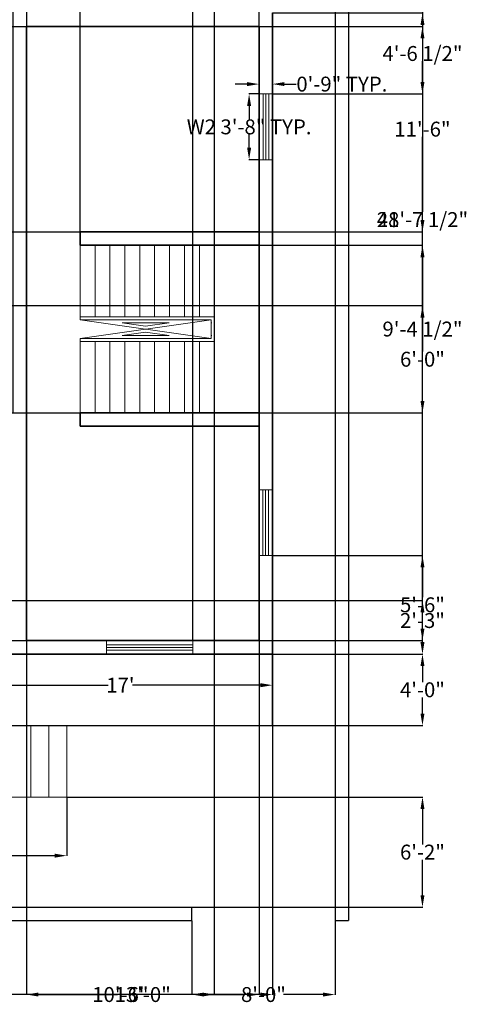
# Model space of a CAD drawing. Units: inches. Extents: x -63 to 800, y 3068 to 4133.
# Tile 3 of 5: x 501 to 800, y 3076 to 3737. Entities that reach past the tile are written whole.
import ezdxf

# ---------------------------------------------------------------- set-up
doc = ezdxf.new("R2010")
doc.units = ezdxf.units.IN
doc.header["$MEASUREMENT"] = 0
for name, color, linetype, lineweight in [('A-ANNO-DIMS', 2, 'Continuous', 13), ('A-FLOR', 7, 'Continuous', 25), ('A-FLOR-STRS', 3, 'Continuous', 18), ('A-GLAZ', 4, 'Continuous', 18), ('A-WALL', 7, 'Continuous', 35), ('A-WALL-SITE', 8, 'Continuous', 30)]:
    doc.layers.add(name, color=color, linetype=linetype, lineweight=lineweight)
doc.styles.get("Standard").update_dxf_attribs({"font": 'arial.ttf'})
doc.dimstyles.get("Standard").update_dxf_attribs({"dimtxt": 10, "dimasz": 8, "dimexe": 0.18, "dimexo": 0.0625, "dimgap": 0.09, "dimtad": 0, "dimtih": 1, "dimtoh": 1, "dimdec": 0, "dimzin": 0, "dimdsep": 46, "dimlunit": 3, "dimtxsty": 'Standard', "dimcen": 0.09, "dimadec": 0, "dimazin": 0, "dimtfac": 1, "dimtdec": 0, "dimtofl": 0, "dimtmove": 0, "dimatfit": 3, "dimfxl": 1, "dimtolj": 1, "dimtzin": 0, "dimarcsym": 0})

# ---------------------------------------------------------------- blocks, each defined once
blk = doc.blocks.new('*D7')
at = {"layer": 'A-ANNO-DIMS', "color": 0, "lineweight": -2, "transparency": 16777216}
for p, q in [((331.31, 3215.25), (331.31, 3175.73)), ((532.31, 3215.25), (532.31, 3175.73)), ((339.31, 3175.91), (415.01, 3175.91)), ((524.31, 3175.91), (448.6, 3175.91))]:
    blk.add_line(p, q, dxfattribs=at)
at = {"layer": 'A-ANNO-DIMS', "color": 0, "transparency": 16777216}
for points in [[(339.31, 3177.24), (339.31, 3174.58), (331.31, 3175.91)], [(524.31, 3177.24), (524.31, 3174.58), (532.31, 3175.91)]]:
    blk.add_solid(points, dxfattribs=at)
at = {"layer": 'Defpoints', "color": 0, "transparency": 16777216}
for p in [(331.31, 3215.31), (532.31, 3215.31), (532.31, 3175.91)]:
    blk.add_point(p, dxfattribs=at)
at = {"layer": 'A-ANNO-DIMS', "color": 0, "transparency": 16777216, "insert": (431.81, 3175.91), "char_height": 10, "attachment_point": 5}
blk.add_mtext('\\A1;16\'-9"', dxfattribs=at)
blk = doc.blocks.new('*D9')
at = {"layer": 'A-ANNO-DIMS', "color": 0, "lineweight": -2, "transparency": 16777216}
for p, q in [((466.31, 3287.37), (466.31, 3290.58)), ((474.31, 3290.4), (560.2, 3290.4)), ((662.31, 3290.4), (576.41, 3290.4)), ((670.31, 3287.37), (670.31, 3290.58))]:
    blk.add_line(p, q, dxfattribs=at)
at = {"layer": 'A-ANNO-DIMS', "color": 0, "transparency": 16777216}
for points in [[(474.31, 3291.73), (474.31, 3289.06), (466.31, 3290.4)], [(662.31, 3291.73), (662.31, 3289.06), (670.31, 3290.4)]]:
    blk.add_solid(points, dxfattribs=at)
at = {"layer": 'Defpoints', "color": 0, "transparency": 16777216}
for p in [(466.31, 3287.31), (670.31, 3290.4), (670.31, 3287.31)]:
    blk.add_point(p, dxfattribs=at)
at = {"layer": 'A-ANNO-DIMS', "color": 0, "transparency": 16777216, "insert": (568.31, 3290.4), "char_height": 10, "attachment_point": 5}
blk.add_mtext("\\A1;17'", dxfattribs=at)
blk = doc.blocks.new('WIN-44')
blk.add_lwpolyline([(0, 0), (0, 44.17), (9, 44.17), (9, 0)], close=True)
for points in [[(2.71, 44.17), (2.71, 0), (6.5, 0), (6.5, 44.17)], [(4.5, 0), (4.5, 44.17)]]:
    blk.add_lwpolyline(points)
blk = doc.blocks.new('WIN-58')
blk.add_lwpolyline([(0, 9), (57.99, 9), (57.99, 0), (0, 0)], close=True)
for points in [[(0, 4.5), (57.99, 4.5), (57.99, 6.29), (0, 6.29)], [(0, 2.51), (57.99, 2.51)]]:
    blk.add_lwpolyline(points)
blk = doc.blocks.new('*D15')
at = {"layer": 'A-ANNO-DIMS', "color": 0, "lineweight": -2, "transparency": 16777216}
for p, q in [((661.25, 3687.44), (654.5, 3687.44)), ((654.68, 3679.44), (654.68, 3670.55)), ((654.68, 3651.26), (654.68, 3660.15)), ((661.25, 3643.26), (654.5, 3643.26))]:
    blk.add_line(p, q, dxfattribs=at)
at = {"layer": 'A-ANNO-DIMS', "color": 0, "transparency": 16777216}
for points in [[(653.35, 3679.44), (656.02, 3679.44), (654.68, 3687.44)], [(653.35, 3651.26), (656.02, 3651.26), (654.68, 3643.26)]]:
    blk.add_solid(points, dxfattribs=at)
at = {"layer": 'Defpoints', "color": 0, "transparency": 16777216}
for p in [(654.68, 3687.44), (661.31, 3687.44), (661.31, 3643.26)]:
    blk.add_point(p, dxfattribs=at)
at = {"layer": 'A-ANNO-DIMS', "color": 0, "transparency": 16777216, "insert": (654.68, 3665.35), "char_height": 10, "attachment_point": 5}
blk.add_mtext('\\A1;W2 3\'-8" TYP.', dxfattribs=at)
blk = doc.blocks.new('*D16')
at = {"layer": 'A-ANNO-DIMS', "color": 0, "lineweight": -2, "transparency": 16777216}
for p, q in [((653.31, 3694.06), (645.31, 3694.06)), ((661.31, 3687.5), (661.31, 3694.24)), ((670.31, 3687.5), (670.31, 3694.24)), ((678.31, 3694.06), (686.31, 3694.06))]:
    blk.add_line(p, q, dxfattribs=at)
at = {"layer": 'A-ANNO-DIMS', "color": 0, "transparency": 16777216}
for points in [[(653.31, 3695.39), (653.31, 3692.73), (661.31, 3694.06)], [(678.31, 3695.39), (678.31, 3692.73), (670.31, 3694.06)]]:
    blk.add_solid(points, dxfattribs=at)
at = {"layer": 'Defpoints', "color": 0, "transparency": 16777216}
for p in [(670.31, 3694.06), (661.31, 3687.44), (670.31, 3687.44)]:
    blk.add_point(p, dxfattribs=at)
at = {"layer": 'A-ANNO-DIMS', "color": 0, "transparency": 16777216, "insert": (716.88, 3694.06), "char_height": 10, "attachment_point": 5}
blk.add_mtext('\\A1;0\'-9" TYP.', dxfattribs=at)
blk = doc.blocks.new('*D22')
at = {"layer": 'A-ANNO-DIMS', "color": 0, "lineweight": -2, "transparency": 16777216}
for p, q in [((616.31, 3132.25), (616.31, 3082.48)), ((712.31, 3132.25), (712.31, 3082.48)), ((624.31, 3082.66), (650.92, 3082.66)), ((704.31, 3082.66), (677.7, 3082.66))]:
    blk.add_line(p, q, dxfattribs=at)
at = {"layer": 'A-ANNO-DIMS', "color": 0, "transparency": 16777216}
for points in [[(624.31, 3083.99), (624.31, 3081.33), (616.31, 3082.66)], [(704.31, 3083.99), (704.31, 3081.33), (712.31, 3082.66)]]:
    blk.add_solid(points, dxfattribs=at)
at = {"layer": 'Defpoints', "color": 0, "transparency": 16777216}
for p in [(616.31, 3132.31), (712.31, 3132.31), (712.31, 3082.66)]:
    blk.add_point(p, dxfattribs=at)
at = {"layer": 'A-ANNO-DIMS', "color": 0, "transparency": 16777216, "insert": (664.31, 3082.66), "char_height": 10, "attachment_point": 5}
blk.add_mtext('\\A1;8\'-0"', dxfattribs=at)
blk = doc.blocks.new('*D33')
at = {"layer": 'A-ANNO-DIMS', "color": 0, "lineweight": -2, "transparency": 16777216}
for p, q in [((532.37, 3215.31), (771.14, 3215.31)), ((770.96, 3207.31), (770.96, 3183.51)), ((770.96, 3149.31), (770.96, 3173.11)), ((616.37, 3141.31), (771.14, 3141.31))]:
    blk.add_line(p, q, dxfattribs=at)
at = {"layer": 'A-ANNO-DIMS', "color": 0, "transparency": 16777216}
for points in [[(769.63, 3207.31), (772.29, 3207.31), (770.96, 3215.31)], [(769.63, 3149.31), (772.29, 3149.31), (770.96, 3141.31)]]:
    blk.add_solid(points, dxfattribs=at)
at = {"layer": 'Defpoints', "color": 0, "transparency": 16777216}
for p in [(532.31, 3215.31), (770.96, 3215.31), (616.31, 3141.31)]:
    blk.add_point(p, dxfattribs=at)
at = {"layer": 'A-ANNO-DIMS', "color": 0, "transparency": 16777216, "insert": (770.96, 3178.31), "char_height": 10, "attachment_point": 5}
blk.add_mtext('\\A1;6\'-2"', dxfattribs=at)
blk = doc.blocks.new('*D34')
at = {"layer": 'A-ANNO-DIMS', "color": 0, "lineweight": -2, "transparency": 16777216}
for p, q in [((142.31, 3522.75), (142.31, 3082.48)), ((670.31, 3263.25), (670.31, 3082.48)), ((150.31, 3082.66), (388.84, 3082.66)), ((662.31, 3082.66), (423.78, 3082.66))]:
    blk.add_line(p, q, dxfattribs=at)
at = {"layer": 'A-ANNO-DIMS', "color": 0, "transparency": 16777216}
for points in [[(150.31, 3083.99), (150.31, 3081.33), (142.31, 3082.66)], [(662.31, 3083.99), (662.31, 3081.33), (670.31, 3082.66)]]:
    blk.add_solid(points, dxfattribs=at)
at = {"layer": 'Defpoints', "color": 0, "transparency": 16777216}
for p in [(142.31, 3522.81), (670.31, 3263.31), (670.31, 3082.66)]:
    blk.add_point(p, dxfattribs=at)
at = {"layer": 'A-ANNO-DIMS', "color": 0, "transparency": 16777216, "insert": (406.31, 3082.66), "char_height": 10, "attachment_point": 5}
blk.add_mtext('\\A1;44\'-0"', dxfattribs=at)
blk = doc.blocks.new('*D35')
at = {"layer": 'A-ANNO-DIMS', "color": 0, "lineweight": -2, "transparency": 16777216}
for p, q in [((640.37, 3894.81), (771.14, 3894.81)), ((770.96, 3886.81), (770.96, 3608.32)), ((770.96, 3319.31), (770.96, 3597.8)), ((670.37, 3311.31), (771.14, 3311.31))]:
    blk.add_line(p, q, dxfattribs=at)
at = {"layer": 'A-ANNO-DIMS', "color": 0, "transparency": 16777216}
for points in [[(769.63, 3886.81), (772.29, 3886.81), (770.96, 3894.81)], [(769.63, 3319.31), (772.29, 3319.31), (770.96, 3311.31)]]:
    blk.add_solid(points, dxfattribs=at)
at = {"layer": 'Defpoints', "color": 0, "transparency": 16777216}
for p in [(640.31, 3894.81), (770.96, 3894.81), (670.31, 3311.31)]:
    blk.add_point(p, dxfattribs=at)
at = {"layer": 'A-ANNO-DIMS', "color": 0, "transparency": 16777216, "insert": (770.96, 3603.06), "char_height": 10, "attachment_point": 5}
blk.add_mtext('\\A1;48\'-7 1/2"', dxfattribs=at)
blk = doc.blocks.new('*D39')
at = {"layer": 'A-ANNO-DIMS', "color": 0, "lineweight": -2, "transparency": 16777216}
for p, q in [((505.31, 3885.75), (505.31, 3082.48)), ((631.31, 3885.75), (631.31, 3082.48)), ((513.31, 3082.66), (551.51, 3082.66)), ((623.31, 3082.66), (585.1, 3082.66))]:
    blk.add_line(p, q, dxfattribs=at)
at = {"layer": 'A-ANNO-DIMS', "color": 0, "transparency": 16777216}
for points in [[(513.31, 3083.99), (513.31, 3081.33), (505.31, 3082.66)], [(623.31, 3083.99), (623.31, 3081.33), (631.31, 3082.66)]]:
    blk.add_solid(points, dxfattribs=at)
at = {"layer": 'Defpoints', "color": 0, "transparency": 16777216}
for p in [(505.31, 3885.81), (631.31, 3885.81), (631.31, 3082.66)]:
    blk.add_point(p, dxfattribs=at)
at = {"layer": 'A-ANNO-DIMS', "color": 0, "transparency": 16777216, "insert": (568.31, 3082.66), "char_height": 10, "attachment_point": 5}
blk.add_mtext('\\A1;10\'-6"', dxfattribs=at)
blk = doc.blocks.new('*D46')
at = {"layer": 'A-ANNO-DIMS', "color": 0, "lineweight": -2, "transparency": 16777216}
for p, q in [((505.31, 3732.75), (505.31, 3082.48)), ((661.31, 3732.75), (661.31, 3082.48)), ((513.31, 3082.66), (566.51, 3082.66)), ((653.31, 3082.66), (600.1, 3082.66))]:
    blk.add_line(p, q, dxfattribs=at)
at = {"layer": 'A-ANNO-DIMS', "color": 0, "transparency": 16777216}
for points in [[(513.31, 3083.99), (513.31, 3081.33), (505.31, 3082.66)], [(653.31, 3083.99), (653.31, 3081.33), (661.31, 3082.66)]]:
    blk.add_solid(points, dxfattribs=at)
at = {"layer": 'Defpoints', "color": 0, "transparency": 16777216}
for p in [(505.31, 3732.81), (661.31, 3732.81), (661.31, 3082.66)]:
    blk.add_point(p, dxfattribs=at)
at = {"layer": 'A-ANNO-DIMS', "color": 0, "transparency": 16777216, "insert": (583.31, 3082.66), "char_height": 10, "attachment_point": 5}
blk.add_mtext('\\A1;13\'-0"', dxfattribs=at)
blk = doc.blocks.new('*D47')
at = {"layer": 'A-ANNO-DIMS', "color": 0, "lineweight": -2, "transparency": 16777216}
for p, q in [((151.37, 3732.81), (771.14, 3732.81)), ((770.96, 3724.81), (770.96, 3669.01)), ((770.96, 3602.81), (770.96, 3658.61)), ((151.37, 3594.81), (771.14, 3594.81))]:
    blk.add_line(p, q, dxfattribs=at)
at = {"layer": 'A-ANNO-DIMS', "color": 0, "transparency": 16777216}
for points in [[(769.63, 3724.81), (772.29, 3724.81), (770.96, 3732.81)], [(769.63, 3602.81), (772.29, 3602.81), (770.96, 3594.81)]]:
    blk.add_solid(points, dxfattribs=at)
at = {"layer": 'Defpoints', "color": 0, "transparency": 16777216}
for p in [(151.31, 3732.81), (770.96, 3732.81), (151.31, 3594.81)]:
    blk.add_point(p, dxfattribs=at)
at = {"layer": 'A-ANNO-DIMS', "color": 0, "transparency": 16777216, "insert": (770.96, 3663.81), "char_height": 10, "attachment_point": 5}
blk.add_mtext('\\A1;11\'-6"', dxfattribs=at)
blk = doc.blocks.new('*D48')
at = {"layer": 'A-ANNO-DIMS', "color": 0, "lineweight": -2, "transparency": 16777216}
for p, q in [((307.37, 3732.81), (771.14, 3732.81)), ((770.96, 3724.81), (770.96, 3608.32)), ((770.96, 3481.31), (770.96, 3597.8)), ((307.37, 3473.31), (771.14, 3473.31))]:
    blk.add_line(p, q, dxfattribs=at)
at = {"layer": 'A-ANNO-DIMS', "color": 0, "transparency": 16777216}
for points in [[(769.63, 3724.81), (772.29, 3724.81), (770.96, 3732.81)], [(769.63, 3481.31), (772.29, 3481.31), (770.96, 3473.31)]]:
    blk.add_solid(points, dxfattribs=at)
at = {"layer": 'Defpoints', "color": 0, "transparency": 16777216}
for p in [(307.31, 3732.81), (770.96, 3732.81), (307.31, 3473.31)]:
    blk.add_point(p, dxfattribs=at)
at = {"layer": 'A-ANNO-DIMS', "color": 0, "transparency": 16777216, "insert": (770.96, 3603.06), "char_height": 10, "attachment_point": 5}
blk.add_mtext('\\A1;21\'-7 1/2"', dxfattribs=at)
blk = doc.blocks.new('*D50')
at = {"layer": 'A-ANNO-DIMS', "color": 0, "lineweight": -2, "transparency": 16777216}
for p, q in [((670.37, 3741.81), (771.14, 3741.81)), ((770.96, 3733.81), (770.96, 3719.88)), ((770.96, 3695.44), (770.96, 3709.36)), ((670.37, 3687.44), (771.14, 3687.44))]:
    blk.add_line(p, q, dxfattribs=at)
at = {"layer": 'A-ANNO-DIMS', "color": 0, "transparency": 16777216}
for points in [[(769.63, 3733.81), (772.29, 3733.81), (770.96, 3741.81)], [(769.63, 3695.44), (772.29, 3695.44), (770.96, 3687.44)]]:
    blk.add_solid(points, dxfattribs=at)
at = {"layer": 'Defpoints', "color": 0, "transparency": 16777216}
for p in [(670.31, 3741.81), (770.96, 3741.81), (670.31, 3687.44)]:
    blk.add_point(p, dxfattribs=at)
at = {"layer": 'A-ANNO-DIMS', "color": 0, "transparency": 16777216, "insert": (770.96, 3714.62), "char_height": 10, "attachment_point": 5}
blk.add_mtext('\\A1;4\'-6 1/2"', dxfattribs=at)
blk = doc.blocks.new('*D53')
at = {"layer": 'A-ANNO-DIMS', "color": 0, "lineweight": -2, "transparency": 16777216}
for p, q in [((541.31, 3594.87), (541.31, 4118.49)), ((549.31, 4118.31), (584.51, 4118.31)), ((653.31, 4118.31), (618.1, 4118.31)), ((661.31, 3594.87), (661.31, 4118.49))]:
    blk.add_line(p, q, dxfattribs=at)
at = {"layer": 'A-ANNO-DIMS', "color": 0, "transparency": 16777216}
for points in [[(549.31, 4119.64), (549.31, 4116.98), (541.31, 4118.31)], [(653.31, 4119.64), (653.31, 4116.98), (661.31, 4118.31)]]:
    blk.add_solid(points, dxfattribs=at)
at = {"layer": 'Defpoints', "color": 0, "transparency": 16777216}
for p in [(661.31, 4118.31), (541.31, 3594.81), (661.31, 3594.81)]:
    blk.add_point(p, dxfattribs=at)
at = {"layer": 'A-ANNO-DIMS', "color": 0, "transparency": 16777216, "insert": (601.31, 4118.31), "char_height": 10, "attachment_point": 5}
blk.add_mtext('\\A1;10\'-0"', dxfattribs=at)
blk = doc.blocks.new('*D54')
at = {"layer": 'A-ANNO-DIMS', "color": 0, "lineweight": -2, "transparency": 16777216}
for p, q in [((661.37, 3585.81), (771.14, 3585.81)), ((770.96, 3577.81), (770.96, 3534.82)), ((770.96, 3481.31), (770.96, 3524.3)), ((661.37, 3473.31), (771.14, 3473.31))]:
    blk.add_line(p, q, dxfattribs=at)
at = {"layer": 'A-ANNO-DIMS', "color": 0, "transparency": 16777216}
for points in [[(769.63, 3577.81), (772.29, 3577.81), (770.96, 3585.81)], [(769.63, 3481.31), (772.29, 3481.31), (770.96, 3473.31)]]:
    blk.add_solid(points, dxfattribs=at)
at = {"layer": 'Defpoints', "color": 0, "transparency": 16777216}
for p in [(661.31, 3585.81), (770.96, 3585.81), (661.31, 3473.31)]:
    blk.add_point(p, dxfattribs=at)
at = {"layer": 'A-ANNO-DIMS', "color": 0, "transparency": 16777216, "insert": (770.96, 3529.56), "char_height": 10, "attachment_point": 5}
blk.add_mtext('\\A1;9\'-4 1/2"', dxfattribs=at)
blk = doc.blocks.new('*D55')
at = {"layer": 'A-ANNO-DIMS', "color": 0, "lineweight": -2, "transparency": 16777216}
for p, q in [((394.37, 3311.31), (771.14, 3311.31)), ((770.96, 3303.31), (770.96, 3292.51)), ((770.96, 3271.31), (770.96, 3282.11)), ((394.37, 3263.31), (771.14, 3263.31))]:
    blk.add_line(p, q, dxfattribs=at)
at = {"layer": 'A-ANNO-DIMS', "color": 0, "transparency": 16777216}
for points in [[(769.63, 3303.31), (772.29, 3303.31), (770.96, 3311.31)], [(769.63, 3271.31), (772.29, 3271.31), (770.96, 3263.31)]]:
    blk.add_solid(points, dxfattribs=at)
at = {"layer": 'Defpoints', "color": 0, "transparency": 16777216}
for p in [(394.31, 3311.31), (770.96, 3311.31), (394.31, 3263.31)]:
    blk.add_point(p, dxfattribs=at)
at = {"layer": 'A-ANNO-DIMS', "color": 0, "transparency": 16777216, "insert": (770.96, 3287.31), "char_height": 10, "attachment_point": 5}
blk.add_mtext('\\A1;4\'-0"', dxfattribs=at)
blk = doc.blocks.new('*D58')
at = {"layer": 'A-ANNO-DIMS', "color": 0, "lineweight": -2, "transparency": 16777216}
for p, q in [((616.98, 3320.37), (616.98, 4118.49)), ((624.98, 4118.31), (653.31, 4118.31)), ((661.31, 3320.37), (661.31, 4118.49)), ((661.31, 4118.31), (669.31, 4118.31))]:
    blk.add_line(p, q, dxfattribs=at)
at = {"layer": 'A-ANNO-DIMS', "color": 0, "transparency": 16777216}
for points in [[(624.98, 4119.64), (624.98, 4116.98), (616.98, 4118.31)], [(653.31, 4119.64), (653.31, 4116.98), (661.31, 4118.31)]]:
    blk.add_solid(points, dxfattribs=at)
at = {"layer": 'Defpoints', "color": 0, "transparency": 16777216}
for p in [(661.31, 4118.31), (616.98, 3320.31), (661.31, 3320.31)]:
    blk.add_point(p, dxfattribs=at)
at = {"layer": 'A-ANNO-DIMS', "color": 0, "transparency": 16777216, "insert": (694.34, 4118.31), "char_height": 10, "attachment_point": 5}
blk.add_mtext('\\A1;3\'-8 1/2"', dxfattribs=at)
blk = doc.blocks.new('*D60')
at = {"layer": 'A-ANNO-DIMS', "color": 0, "lineweight": -2, "transparency": 16777216}
for p, q in [((670.26, 3377.44), (771.14, 3377.44)), ((770.96, 3369.44), (770.96, 3349.57)), ((770.96, 3319.31), (770.96, 3339.18)), ((670.37, 3311.31), (771.14, 3311.31))]:
    blk.add_line(p, q, dxfattribs=at)
at = {"layer": 'A-ANNO-DIMS', "color": 0, "transparency": 16777216}
for points in [[(769.63, 3369.44), (772.29, 3369.44), (770.96, 3377.44)], [(769.63, 3319.31), (772.29, 3319.31), (770.96, 3311.31)]]:
    blk.add_solid(points, dxfattribs=at)
at = {"layer": 'Defpoints', "color": 0, "transparency": 16777216}
for p in [(670.2, 3377.44), (770.96, 3377.44), (670.31, 3311.31)]:
    blk.add_point(p, dxfattribs=at)
at = {"layer": 'A-ANNO-DIMS', "color": 0, "transparency": 16777216, "insert": (770.96, 3344.38), "char_height": 10, "attachment_point": 5}
blk.add_mtext('\\A1;5\'-6"', dxfattribs=at)
blk = doc.blocks.new('*D62')
at = {"layer": 'A-ANNO-DIMS', "color": 0, "lineweight": -2, "transparency": 16777216}
for p, q in [((478.66, 4118.31), (470.66, 4118.31)), ((486.66, 3473.37), (486.66, 4118.49)), ((496.31, 3473.37), (496.31, 4118.49)), ((504.31, 4118.31), (512.31, 4118.31))]:
    blk.add_line(p, q, dxfattribs=at)
at = {"layer": 'A-ANNO-DIMS', "color": 0, "transparency": 16777216}
for points in [[(478.66, 4119.64), (478.66, 4116.98), (486.66, 4118.31)], [(504.31, 4119.64), (504.31, 4116.98), (496.31, 4118.31)]]:
    blk.add_solid(points, dxfattribs=at)
at = {"layer": 'Defpoints', "color": 0, "transparency": 16777216}
for p in [(496.31, 4118.31), (486.66, 3473.31), (496.31, 3473.31)]:
    blk.add_point(p, dxfattribs=at)
at = {"layer": 'A-ANNO-DIMS', "color": 0, "transparency": 16777216, "insert": (537.34, 4118.31), "char_height": 10, "attachment_point": 5}
blk.add_mtext('\\A1;0\'-9 1/2"', dxfattribs=at)
blk = doc.blocks.new('*D63')
at = {"layer": 'A-ANNO-DIMS', "color": 0, "lineweight": -2, "transparency": 16777216}
for p, q in [((190.37, 3545.31), (771.14, 3545.31)), ((770.96, 3537.31), (770.96, 3514.51)), ((770.96, 3481.31), (770.96, 3504.11)), ((190.37, 3473.31), (771.14, 3473.31))]:
    blk.add_line(p, q, dxfattribs=at)
at = {"layer": 'A-ANNO-DIMS', "color": 0, "transparency": 16777216}
for points in [[(769.63, 3537.31), (772.29, 3537.31), (770.96, 3545.31)], [(769.63, 3481.31), (772.29, 3481.31), (770.96, 3473.31)]]:
    blk.add_solid(points, dxfattribs=at)
at = {"layer": 'Defpoints', "color": 0, "transparency": 16777216}
for p in [(190.31, 3545.31), (770.96, 3545.31), (190.31, 3473.31)]:
    blk.add_point(p, dxfattribs=at)
at = {"layer": 'A-ANNO-DIMS', "color": 0, "transparency": 16777216, "insert": (770.96, 3509.31), "char_height": 10, "attachment_point": 5}
blk.add_mtext('\\A1;6\'-0"', dxfattribs=at)
blk = doc.blocks.new('*D71')
at = {"layer": 'A-ANNO-DIMS', "color": 0, "lineweight": -2, "transparency": 16777216}
for p, q in [((358.37, 3347.31), (771.14, 3347.31)), ((770.96, 3339.31), (770.96, 3339.01)), ((770.96, 3328.31), (770.96, 3328.61)), ((356.37, 3320.31), (771.14, 3320.31))]:
    blk.add_line(p, q, dxfattribs=at)
at = {"layer": 'A-ANNO-DIMS', "color": 0, "transparency": 16777216}
for points in [[(769.63, 3339.31), (772.29, 3339.31), (770.96, 3347.31)], [(769.63, 3328.31), (772.29, 3328.31), (770.96, 3320.31)]]:
    blk.add_solid(points, dxfattribs=at)
at = {"layer": 'Defpoints', "color": 0, "transparency": 16777216}
for p in [(358.31, 3347.31), (356.31, 3320.31), (770.96, 3320.31)]:
    blk.add_point(p, dxfattribs=at)
at = {"layer": 'A-ANNO-DIMS', "color": 0, "transparency": 16777216, "insert": (770.96, 3333.81), "char_height": 10, "attachment_point": 5}
blk.add_mtext('\\A1;2\'-3"', dxfattribs=at)

msp = doc.modelspace()

# ---------------------------------------------------------------- linework, layer by layer
at = {"layer": 'A-FLOR'}
msp.add_line((466.31, 3263.31), (670.31, 3263.31), dxfattribs=at)
at = {"layer": 'A-FLOR-STRS'}
for p, q in [((541.31, 3535.81), (541.31, 3585.81)), ((551.31, 3537.81), (551.31, 3585.81)), ((561.31, 3537.81), (561.31, 3585.81)), ((571.31, 3537.81), (571.31, 3585.81)), ((581.31, 3537.81), (581.31, 3585.81)), ((591.31, 3537.81), (591.31, 3585.81)), ((601.31, 3537.81), (601.31, 3585.81)), ((611.31, 3537.81), (611.31, 3585.81)), ((621.31, 3537.81), (621.31, 3585.81)), ((631.31, 3537.81), (631.31, 3585.81)), ((541.31, 3537.81), (631.31, 3537.81)), ((631.31, 3537.81), (631.31, 3521.26)), ((541.31, 3535.81), (629.31, 3535.81)), ((541.31, 3535.81), (629.31, 3523.26)), ((629.31, 3535.81), (541.31, 3523.31)), ((569.49, 3533.81), (585.22, 3531.57)), ((569.49, 3533.81), (601.01, 3533.81)), ((601.01, 3533.81), (585.22, 3531.57)), ((629.31, 3535.81), (629.31, 3523.26)), ((629.59, 3533.83), (629.31, 3533.79)), ((585.22, 3527.53), (569.49, 3525.29)), ((601.01, 3525.27), (569.49, 3525.29)), ((585.22, 3527.53), (601.01, 3525.27)), ((629.31, 3525.28), (629.59, 3525.24)), ((629.31, 3525.26), (629.31, 3525.26)), ((541.31, 3521.31), (541.31, 3523.31)), ((629.31, 3523.26), (541.31, 3523.31)), ((541.31, 3473.31), (541.31, 3521.31)), ((631.31, 3521.26), (541.31, 3521.31)), ((551.31, 3473.31), (551.31, 3521.31)), ((561.31, 3473.31), (561.31, 3521.31)), ((571.31, 3473.31), (571.31, 3521.31)), ((581.31, 3473.31), (581.31, 3521.31)), ((591.31, 3473.31), (591.31, 3521.31)), ((601.31, 3473.31), (601.31, 3521.31)), ((611.31, 3473.31), (611.31, 3521.31)), ((621.31, 3473.31), (621.31, 3521.31)), ((629.31, 3521.26), (629.31, 3521.26)), ((631.31, 3523.26), (631.31, 3523.26)), ((631.31, 3473.31), (631.31, 3521.31)), ((508.31, 3263.31), (508.31, 3215.31)), ((520.31, 3263.31), (520.31, 3215.31)), ((532.31, 3263.31), (532.31, 3215.31)), ((331.31, 3215.31), (532.31, 3215.31))]:
    msp.add_line(p, q, dxfattribs=at)
at = {"layer": 'A-WALL'}
for p, q in [((670.31, 3741.81), (670.31, 3263.31)), ((505.31, 3732.81), (505.31, 3594.81)), ((505.31, 3732.81), (661.31, 3732.81)), ((661.31, 3732.81), (661.31, 3594.81)), ((541.31, 3594.81), (661.31, 3594.81)), ((505.31, 3585.81), (505.31, 3473.31)), ((541.31, 3585.81), (661.31, 3585.81)), ((661.31, 3585.81), (661.31, 3473.31)), ((541.31, 3473.31), (661.31, 3473.31)), ((505.31, 3464.31), (505.31, 3320.31)), ((541.31, 3464.31), (661.31, 3464.31)), ((661.31, 3464.31), (661.31, 3320.31)), ((505.31, 3320.31), (661.31, 3320.31)), ((466.31, 3311.31), (670.31, 3311.31))]:
    msp.add_line(p, q, dxfattribs=at)
for points in [[(505.31, 3585.81), (505.31, 3596.81)], [(541.31, 3594.81), (541.31, 3585.81)], [(505.31, 3464.31), (505.31, 3464.31), (505.31, 3475.31)], [(541.31, 3473.31), (541.31, 3464.31)]]:
    msp.add_lwpolyline(points, dxfattribs=at)
at = {"layer": 'A-WALL-SITE'}
for p, q in [((721.31, 4068.66), (721.31, 3132.31)), ((712.31, 4059.66), (712.31, 3132.31)), ((121.31, 3141.31), (616.31, 3141.31)), ((121.31, 3132.31), (616.31, 3132.31)), ((712.31, 3132.31), (721.31, 3132.31))]:
    msp.add_line(p, q, dxfattribs=at)
for points in [[(616.31, 3132.31), (616.31, 3141.31)], [(712.31, 3141.31), (712.31, 3141.31), (712.31, 3132.31)]]:
    msp.add_lwpolyline(points, dxfattribs=at)

# ---------------------------------------------------------------- block references
at = {"layer": 'A-GLAZ'}
for name, p in [('WIN-44', (661.31, 3643.26)), ('WIN-44', (661.2, 3377.44)), ('WIN-58', (558.99, 3311.31))]:
    msp.add_blockref(name, p, dxfattribs=at)

# ---------------------------------------------------------------- dimensions: what is measured, and where the dimension line sits
at = {"layer": 'A-ANNO-DIMS'}
for base, p1, p2, override, picture, middle in [((496.3095, 4118.3113), (486.6577, 3473.3102), (496.3095, 3473.3102), {"dimdec": 1, "dimlfac": 1, "dimrnd": 0, "dimzin": 1, "dimdsep": 46, "dimlunit": 4, "dimfrac": 2}, '*D62', (537.3415, 4118.3113)), ((661.31, 4118.31), (616.98, 3320.31), (661.31, 3320.31), {"dimdec": 1, "dimlfac": 1, "dimrnd": 0, "dimzin": 1, "dimdsep": 46, "dimlunit": 4, "dimfrac": 2}, '*D58', (694.34, 4118.31)), ((661.31, 4118.31), (541.31, 3594.81), (661.31, 3594.81), {"dimdec": 1, "dimlfac": 1, "dimrnd": 0, "dimzin": 1, "dimdsep": 46, "dimlunit": 4, "dimfrac": 2}, '*D53', (601.31, 4118.31)), ((631.31, 3082.66), (505.31, 3885.81), (631.31, 3885.81), {"dimdec": 1, "dimlfac": 1, "dimrnd": 0, "dimzin": 1, "dimdsep": 46, "dimlunit": 4, "dimfrac": 2}, '*D39', (568.31, 3082.66)), ((661.31, 3082.66), (505.31, 3732.81), (661.31, 3732.81), {"dimdec": 1, "dimlfac": 1, "dimrnd": 0, "dimzin": 1, "dimdsep": 46, "dimlunit": 4, "dimfrac": 2}, '*D46', (583.31, 3082.66)), ((670.31, 3082.66), (142.31, 3522.81), (670.31, 3263.31), {"dimdec": 1, "dimlfac": 1, "dimrnd": 0, "dimzin": 1, "dimdsep": 46, "dimlunit": 4, "dimfrac": 2}, '*D34', (406.31, 3082.66)), ((670.31, 3290.4), (466.31, 3287.31), (670.31, 3287.31), {"dimclrd": 0, "dimclre": 0, "dimclrt": 0}, '*D9', (568.31, 3290.4)), ((532.31, 3175.91), (331.31, 3215.31), (532.31, 3215.31), {"dimclrd": 0, "dimclre": 0, "dimclrt": 0}, '*D7', (431.81, 3175.91)), ((712.31, 3082.66), (616.31, 3132.31), (712.31, 3132.31), {"dimdec": 1, "dimlfac": 1, "dimrnd": 0, "dimzin": 1, "dimdsep": 46, "dimlunit": 4, "dimfrac": 2}, '*D22', (664.31, 3082.66))]:
    dim = msp.add_linear_dim(base=base, p1=p1, p2=p2, dimstyle='Standard', override=override, dxfattribs=at)
    dim.commit()
    dim.dimension.update_dxf_attribs({"geometry": picture, "text_midpoint": middle})
for base, p1, p2, picture, middle in [((770.96, 3894.81), (670.31, 3311.31), (640.31, 3894.81), '*D35', (770.96, 3603.06)), ((770.96, 3741.81), (670.31, 3687.44), (670.31, 3741.81), '*D50', (770.96, 3714.62)), ((770.96, 3732.81), (151.31, 3594.81), (151.31, 3732.81), '*D47', (770.96, 3663.81)), ((770.96, 3732.81), (307.31, 3473.31), (307.31, 3732.81), '*D48', (770.96, 3603.06)), ((770.96, 3585.81), (661.31, 3473.31), (661.31, 3585.81), '*D54', (770.96, 3529.56)), ((770.96, 3545.31), (190.31, 3473.31), (190.31, 3545.31), '*D63', (770.96, 3509.31)), ((770.96, 3377.44), (670.31, 3311.31), (670.2, 3377.44), '*D60', (770.96, 3344.38)), ((770.96, 3320.31), (358.31, 3347.31), (356.31, 3320.31), '*D71', (770.96, 3333.81)), ((770.96, 3311.31), (394.31, 3263.31), (394.31, 3311.31), '*D55', (770.96, 3287.31)), ((770.96, 3215.31), (616.31, 3141.31), (532.31, 3215.31), '*D33', (770.96, 3178.31))]:
    dim = msp.add_linear_dim(base=base, p1=p1, p2=p2, angle=90, dimstyle='Standard', override={"dimdec": 1, "dimlfac": 1, "dimrnd": 0, "dimzin": 1, "dimdsep": 46, "dimlunit": 4, "dimfrac": 2}, dxfattribs=at)
    dim.commit()
    dim.dimension.update_dxf_attribs({"geometry": picture, "text_midpoint": middle})
dim = msp.add_linear_dim(base=(670.31, 3694.06), p1=(661.31, 3687.44), p2=(670.31, 3687.44), text='<> TYP.', dimstyle='Standard', override={"dimdec": 1, "dimlfac": 1, "dimrnd": 0, "dimzin": 1, "dimdsep": 46, "dimlunit": 4, "dimfrac": 2}, dxfattribs=at)
dim.commit()
dim.dimension.update_dxf_attribs({"geometry": '*D16', "text_midpoint": (716.88, 3694.06)})
dim = msp.add_linear_dim(base=(654.68, 3687.44), p1=(661.31, 3643.26), p2=(661.31, 3687.44), angle=90, text='W2 <> TYP.', dimstyle='Standard', override={"dimdec": 1, "dimlfac": 1, "dimrnd": 0, "dimzin": 1, "dimdsep": 46, "dimlunit": 4, "dimfrac": 2}, dxfattribs=at)
dim.commit()
dim.dimension.update_dxf_attribs({"geometry": '*D15', "text_midpoint": (654.68, 3665.35)})

doc.saveas('drawing.dxf')
